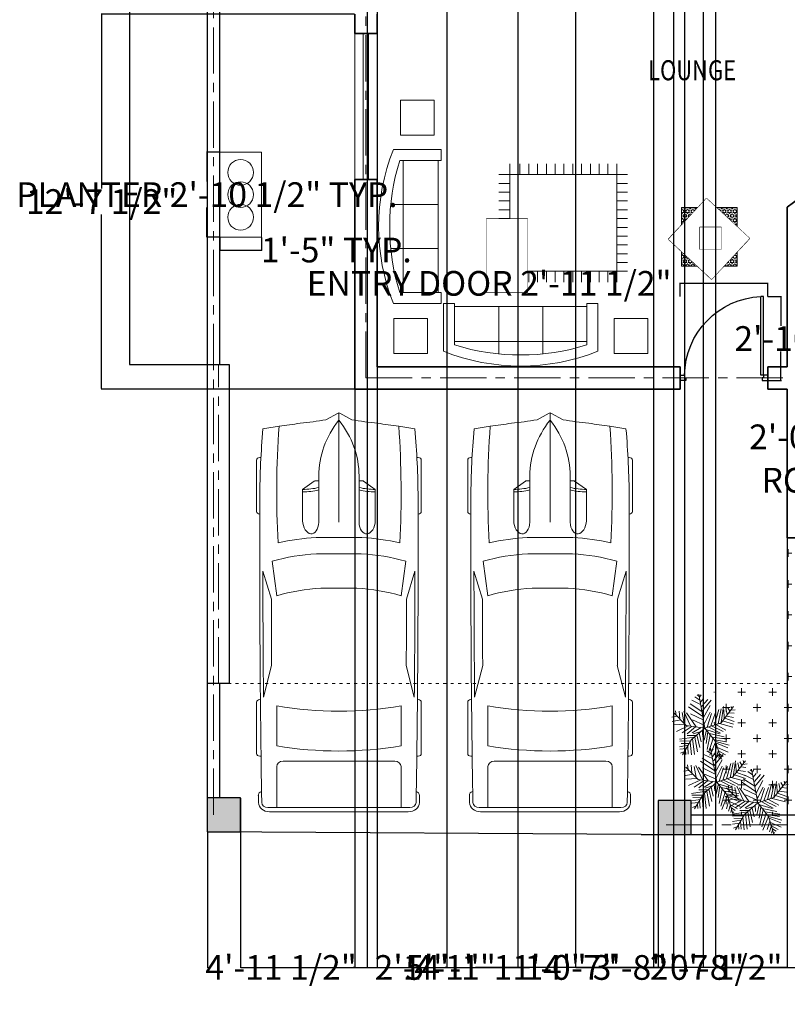
# Model space of a CAD drawing. Units: inches. Extents: x 541 to 1172, y -20 to 887.
# Tile 1 of 8: x 541 to 851, y -20 to 378. Entities that reach past the tile are written whole.
import ezdxf

# ---------------------------------------------------------------- set-up
doc = ezdxf.new("R2010")
doc.units = ezdxf.units.IN
doc.header["$MEASUREMENT"] = 0
doc.set_wipeout_variables(frame=1)
doc.linetypes.add('ACAD_ISO03W100', pattern=[30, 12, -18])
doc.linetypes.add('CENTER', pattern=[50.8, 31.75, -6.35, 6.35, -6.35])
doc.layers.get('0').update_dxf_attribs({"color": 70})
for name, color, linetype, lineweight in [('A-ANNO-DIMS', 2, 'Continuous', 18), ('A-AREA-IDEN', 7, 'Continuous', 20), ('A-DOOR', 4, 'Continuous', 25), ('A-FURN', 30, 'Continuous', 18), ('A-ROOF-OVHD', 8, 'ACAD_ISO03W100', 18), ('A-WALL-CNTR', 1, 'CENTER', 13), ('C-PKNG-VEHI', 8, 'Continuous', 18), ('C-PROP', 7, 'Continuous', 25), ('L-PLNT', 70, 'Continuous', 18), ('L-PLNT-PATT', 70, 'Continuous', 13), ('L-SITE-PATT', 252, 'Continuous', 13), ('L-SITE-WALL', 7, 'Continuous', 30), ('WALL', 7, 'Continuous', 35), ('WINDOW', 2, 'Continuous', 18)]:
    doc.layers.add(name, color=color, linetype=linetype, lineweight=lineweight)
doc.styles.get("Standard").update_dxf_attribs({"font": 'arial.ttf'})
doc.styles.add('YQ_DIM', font='SUPEROS.SHX', dxfattribs={"width": 0.8, "bigfont": 'HZDX.SHX'})
doc.dimstyles.get("Standard").update_dxf_attribs({"dimtxt": 10, "dimasz": 0.18, "dimexe": 0.18, "dimexo": 0.0625, "dimgap": 0.09, "dimtad": 0, "dimtih": 1, "dimtoh": 1, "dimdec": 1, "dimzin": 0, "dimdsep": 46, "dimlunit": 4, "dimtxsty": 'Standard', "dimcen": 0.09, "dimadec": 0, "dimazin": 0, "dimtfac": 1, "dimtdec": 1, "dimtofl": 0, "dimtmove": 0, "dimatfit": 3, "dimfxl": 1, "dimtolj": 1, "dimtzin": 0, "dimarcsym": 0})

# ---------------------------------------------------------------- blocks, each defined once
blk = doc.blocks.new('*D3')
at = {"layer": 'A-ANNO-DIMS', "color": 0, "lineweight": -2, "transparency": 16777216}
for p, q in [((616.57, 829.68), (585.07, 829.68)), ((585.25, 829.5), (585.25, 539.38)), ((585.25, 238.86), (585.25, 528.98)), ((621.57, 238.68), (585.07, 238.68))]:
    blk.add_line(p, q, dxfattribs=at)
for points in [[(585.22, 829.5), (585.28, 829.5), (585.25, 829.68)], [(585.22, 238.86), (585.28, 238.86), (585.25, 238.68)]]:
    blk.add_solid(points, dxfattribs=at)
at = {"layer": 'Defpoints', "color": 0, "lineweight": -2, "transparency": 16777216}
for p in [(616.64, 829.68), (585.25, 238.68), (621.64, 238.68)]:
    blk.add_point(p, dxfattribs=at)
at = {"layer": 'A-ANNO-DIMS', "color": 0, "transparency": 16777216, "insert": (585.25, 534.18), "char_height": 10, "attachment_point": 5}
blk.add_mtext('\\A1;49\'-3"', dxfattribs=at)
blk = doc.blocks.new('*U5')
for p, q in [((21.1, 37.41), (21.1, 36.83)), ((46.55, 38.89), (22.35, 38.89)), ((47.8, 37.39), (47.8, 37.41)), ((135.45, 37.07), (135.45, 37.41)), ((136.7, 38.89), (160.9, 38.89)), ((162.15, 37.41), (162.15, 36.77)), ((87.99, 31.87), (74.76, 35.92)), ((134.31, 35.6), (119.29, 31.78)), ((186.47, -33.5), (186.47, 33.5)), ((188.4, -32.76), (188.4, 32.76)), ((70.03, 31.54), (86.41, 29.35)), ((138.42, 29.35), (157.25, 29.35)), ((186.47, 29.35), (167.01, 29.35)), ((164.52, 26.39), (164.52, -26.39)), ((32.27, 11.63), (36.13, 17.17)), ((36.13, 17.17), (50.94, 17.17)), ((29.77, 9.51), (51.68, 9.51)), ((32.12, 9.51), (32.12, 11.15)), ((58.92, -10.77), (58.92, 10.77)), ((66.55, -10.53), (66.55, 10.53)), ((186.47, -10.53), (186.47, 10.53)), ((3.27, 6.13), (0.1, 0.41)), ((82.74, 8.5), (82.74, -8.5)), ((0, 0), (51.68, 0)), ((0.1, -0.41), (3.27, -6.13)), ((29.77, -9.51), (51.68, -9.51)), ((32.12, -9.51), (32.12, -11.15)), ((32.27, -11.63), (36.13, -17.17)), ((36.13, -17.17), (50.94, -17.17)), ((86.41, -29.35), (70.03, -31.54)), ((87.99, -31.87), (74.76, -35.92)), ((134.31, -35.6), (119.29, -31.78)), ((157.25, -29.35), (138.42, -29.35)), ((167.01, -29.35), (186.47, -29.35)), ((21.1, -37.41), (21.1, -36.83)), ((135.45, -37.07), (135.45, -37.41)), ((162.15, -37.41), (162.15, -36.77)), ((46.55, -38.89), (22.35, -38.89)), ((47.8, -37.39), (47.8, -37.41)), ((136.7, -38.89), (160.9, -38.89))]:
    blk.add_line(p, q)
for centre, major_axis, ratio, start_param, end_param in [((41.19, -490.86), (0, 528.23), 0.842304, 0.00281, 0.075598), ((22.35, 37.41), (0, -1.48), 0.842304, 3.141593, 4.712389), ((64.48, -10555.62), (0, 10593.03), 0.842304, -0.013397, 0.002797), ((46.55, 37.41), (0, 1.48), 0.842304, -1.570796, 0), ((136.7, 37.41), (0, -1.48), 0.842304, 3.141593, 4.712389), ((160.9, 37.41), (0, 1.48), 0.842304, -1.570796, 0), ((180.63, 35.84), (0, 2.22), 0.842304, -0.013017, 1.249894), ((64.48, -10556.36), (0, 10595.31), 0.842304, -0.013397, -0.013017), ((183.98, 32.76), (0, -5.25), 0.842304, 1.570796, 3.128196), ((266.03, -27.52), (0, 313.31), 0.842304, 1.367076, 1.39176), ((64.48, -10555.62), (0, -10591.55), 0.842304, 3.133765, 3.140441), ((183.98, 33.5), (0, -2.96), 0.842304, 1.570796, 3.128196), ((259.18, -27.52), (0, -305.3), 0.842304, 4.528606, 4.561838), ((37.47, -593.96), (0, -623.33), 0.842304, 3.096046, 3.200911), ((134.4, 5.39), (0, -89.78), 0.842304, 4.449482, 4.652344), ((135.29, 5.39), (0, 81.77), 0.842304, 1.245306, 1.50788), ((149.6, 2.8), (0, -79.58), 0.842304, 4.372215, 4.640744), ((95.79, -3666.35), (0, -3698.24), 0.842304, 3.134049, 3.144098), ((17.08, 0), (0, 147.02), 0.842304, 4.511394, 4.913384), ((35.91, 0), (0, 147.02), 0.842304, 4.511394, 4.913384), ((167.01, 26.39), (0, 2.96), 0.842304, 0, 1.570796), ((-204.49, 52.4), (0, -250.96), 0.842304, 1.385369, 1.434372), ((13.04, 17.01), (0, 27.42), 0.842304, 4.435146, 4.718221), ((14.2, 17.01), (0, 27.42), 0.842304, 4.435146, 4.718221), ((50.79, 13.34), (6.34, -0.36), 0.603834, -1.395552, 1.581315), ((29.77, -46.66), (0, 56.17), 0.842304, 0, 0.590319), ((32.75, 11.15), (0, 0.74), 0.842304, 0.879714, 1.570796), ((0.62, 0), (0, -0.74), 0.842304, 4.131459, 5.293319), ((29.77, 46.66), (0, 56.17), 0.842304, 2.551274, 3.141593), ((-204.49, -52.4), (0, 250.96), 0.842304, -1.434372, -1.385369), ((149.6, -2.8), (0, -79.58), 0.842304, -1.499151, -1.230623), ((32.75, -11.15), (0, -0.74), 0.842304, 4.712389, 5.403472), ((13.04, -17.01), (0, -27.42), 0.842304, 1.564964, 1.848039), ((14.2, -17.01), (0, -27.42), 0.842304, 1.564964, 1.848039), ((134.4, -5.39), (0, -89.78), 0.842304, -1.510751, -1.307889), ((135.29, -5.39), (0, -81.77), 0.842304, -1.50788, -1.245306), ((259.18, 27.52), (0, 305.3), 0.842304, 1.721348, 1.754579), ((167.01, -26.39), (0, -2.96), 0.842304, 4.712389, 6.283185), ((266.03, 27.52), (0, 313.31), 0.842304, 1.749832, 1.774517), ((37.47, 593.96), (0, -623.33), 0.842304, -0.059319, 0.045547), ((95.79, 3666.35), (0, -3698.24), 0.842304, -0.002505, 0.007544), ((41.19, 490.86), (0, -528.23), 0.842304, -0.075598, -0.00281), ((64.48, 10555.62), (0, 10593.03), 0.842304, 3.138796, 3.15499), ((64.48, 10555.62), (0, -10591.55), 0.842304, 0.001152, 0.007828), ((180.63, -35.84), (0, -2.22), 0.842304, -1.249894, 0.013017), ((183.98, -33.5), (0, 2.96), 0.842304, 3.15499, 4.712389), ((183.98, -32.76), (0, -5.25), 0.842304, 0.013397, 1.570796), ((22.35, -37.41), (0, 1.48), 0.842304, 1.570796, 3.141593), ((46.55, -37.41), (0, -1.48), 0.842304, 0, 1.570796), ((136.7, -37.41), (0, -1.48), 0.842304, -1.570796, 0), ((160.9, -37.41), (0, 1.48), 0.842304, 3.141593, 4.712389), ((64.48, 10556.36), (0, 10595.31), 0.842304, 3.15461, 3.15499)]:
    blk.add_ellipse(centre, major_axis=major_axis, ratio=ratio, start_param=start_param, end_param=end_param)
at = {"extrusion": (0, 0, -1)}
blk.add_ellipse((50.79, -13.34), major_axis=(6.34, 0.36), ratio=0.603834, start_param=-1.395552, end_param=1.581315, dxfattribs=at)
blk = doc.blocks.new('*U7')
for p, q in [((-8.737, 47.138), (-17.069, 52.711)), ((-10.186, 53.64), (-13.084, 55.962)), ((0, 0), (-10.5, 57)), ((-9.099, 51.782), (-6.563, 55.962)), ((-3.665, 19.273), (-27.574, 35.527)), ((-5.114, 28.097), (-24.676, 40.636)), ((-7.288, 39.707), (-21.778, 46.673)), ((-7.65, 43.423), (-2.578, 49.46)), ((-5.839, 35.992), (4.667, 48.067)), ((-5.114, 27.632), (10.463, 46.673)), ((-2.941, 16.486), (8.652, 37.85)), ((27, 9), (48, 36)), ((27.127, 9.056), (31.112, 35.992)), ((38.719, 34.134), (41.979, 28.561)), ((44.153, 36.456), (45.239, 32.741)), ((-47.498, 19.737), (-55.83, 18.344)), ((-31.5, 4.5), (-52.5, 25.5)), ((-48.585, 21.131), (-49.309, 29.026)), ((-43.513, 28.561), (-42.427, 15.558)), ((-38.442, 26.239), (-34.819, 7.663)), ((-35.544, 28.097), (-24.314, 3.947)), ((-14.533, 2.09), (-30.834, 25.31)), ((-24.314, 23.917), (-2.941, 13.7)), ((-1.129, 6.734), (9.014, 26.704)), ((3.942, 1.625), (11.187, 24.381)), ((10.101, 3.483), (17.708, 26.239)), ((16.259, 5.805), (23.142, 31.348)), ((22.055, 7.198), (27.489, 32.277)), ((31.836, 30.883), (32.561, 16.486)), ((35.096, 32.741), (37.27, 22.524)), ((36.183, 19.737), (48.137, 17.88)), ((40.53, 25.775), (48.862, 24.846)), ((43.791, 29.954), (51.036, 30.883)), ((-40.615, 13.7), (-55.105, 10.913)), ((-33.37, 6.269), (-52.207, 5.34)), ((-28.299, 3.483), (-47.86, -5.805)), ((-21.416, 3.018), (-38.079, -8.128)), ((0, 0), (-31.5, 4.5)), ((-15.982, 2.09), (-30.11, -9.521)), ((0, 0), (-22.5, -19.5)), ((-6.563, 1.161), (-21.416, -8.128)), ((-20.691, 13.7), (-1.129, 4.876)), ((0, 0), (27, 9)), ((0, 0), (18, -22.5)), ((6.478, 1.625), (26.04, -8.592)), ((11.187, 3.483), (30.749, -5.805)), ((18.07, 5.805), (35.096, -3.483)), ((24.229, 7.663), (46.688, 1.625)), ((29.662, 12.307), (48.137, 6.269)), ((33.285, 16.486), (48.862, 10.913)), ((-17.431, -15.094), (-42.789, -18.809)), ((-15.257, -12.772), (-30.11, -12.772)), ((-6.563, -5.805), (-19.967, -9.985)), ((-17.069, -15.094), (-12.721, -40.172)), ((-13.446, -11.378), (-8.737, -32.741)), ((-9.461, -8.592), (-6.201, -23.453)), ((-4.752, -3.483), (-3.665, -14.629)), ((2.493, -3.019), (-1.491, -20.202)), ((1.769, -2.555), (24.229, -9.521)), ((5.029, -6.27), (2.131, -25.775)), ((9.014, -11.378), (3.58, -35.992)), ((7.565, -9.056), (32.198, -14.629)), ((12.274, -15.094), (36.907, -18.809)), ((-28.299, -29.026), (-42.789, -31.348)), ((-24.314, -21.596), (-42.427, -22.06)), ((-26.849, -26.24), (-40.253, -25.775)), ((-22.5, -19.5), (-37.5, -45)), ((-29.023, -30.884), (-27.936, -43.887)), ((-25.038, -23.918), (-22.865, -45.281)), ((-20.691, -18.345), (-17.793, -44.352)), ((14.085, -16.951), (6.478, -40.172)), ((18.07, -22.524), (8.289, -45.745)), ((20.244, -30.419), (15.897, -44.816)), ((16.259, -19.738), (36.183, -22.989)), ((18, -22.5), (27, -52.5)), ((18.433, -22.524), (40.53, -29.026)), ((19.157, -25.311), (38.719, -33.206)), ((21.331, -32.741), (39.081, -40.636)), ((-30.834, -34.135), (-42.427, -35.528)), ((-34.457, -39.708), (-40.978, -42.494)), ((-32.646, -36.921), (-31.921, -44.352)), ((22.78, -37.85), (19.519, -48.532)), ((22.78, -38.314), (34.372, -44.816)), ((24.591, -45.745), (23.142, -50.854)), ((24.591, -43.423), (30.749, -47.603)), ((26.764, -49.925), (28.213, -50.854))]:
    blk.add_line(p, q)
blk = doc.blocks.new('Sofa - Roundback 7 ft.')
for p, q in [((-12.00002, -32.4421), (-12.00003, -6.5971)), ((11.99997, -32.4421), (11.99998, -6.5971)), ((-36.000027, -34), (-36.000027, -11.4696)), ((-35.999844, -13.3819), (35.9998, -13.3819)), ((35.99998, -34), (35.99998, -11.4696)), ((-36.000027, -32.4421), (35.99998, -32.4421))]:
    blk.add_line(p, q)
for points in [[(-36.000027, -34), (-42.000027, -34), (-42.000027, -8)], [(41.99998, -8), (41.99998, -34), (35.99998, -34)]]:
    blk.add_lwpolyline(points)
for centre, radius, start, end in [((0, -114.25), 114.25, 68.43141, 111.5686), ((-0.00001, -127.1968), 121.1968, 72.72033, 107.2797)]:
    blk.add_arc(centre, radius, start, end)
blk = doc.blocks.new('DR_D01')
at = {"lineweight": -2}
for p, q in [((-0.45, 0.93), (-0.42, 0.93)), ((-0.45, 0.03), (-0.45, 0.93)), ((-0.42, 0.03), (-0.42, 0.93)), ((-0.5, 0.03), (-0.42, 0.03)), ((-0.5, 0.03), (-0.5, -0.03)), ((-0.45, 0.03), (-0.45, 0)), ((-0.45, 0), (-0.435, 0)), ((-0.435, 0), (-0.435, -0.03)), ((0.435, 0), (0.435, -0.03)), ((0.45, 0), (0.435, 0)), ((0.45, 0.03), (0.45, 0)), ((0.5, 0.03), (0.45, 0.03)), ((0.5, -0.03), (0.5, 0.03)), ((-0.435, -0.03), (-0.5, -0.03)), ((0.435, -0.03), (0.5, -0.03))]:
    blk.add_line(p, q, dxfattribs=at)
blk.add_arc((-0.46, 0.021), 0.91, 0.5915, 87.4664, dxfattribs=at)
blk = doc.blocks.new('WD_WIN4')
at = {"lineweight": -2}
for p, q in [((-0.5, 0.5), (0.5, 0.5)), ((-0.5, 0.12), (0.5, 0.12)), ((-0.5, -0.12), (0.5, -0.12)), ((-0.5, -0.5), (0.5, -0.5))]:
    blk.add_line(p, q, dxfattribs=at)
blk = doc.blocks.new('PLANTER-THREE-ROUND')
blk.add_lwpolyline([(34.49, 16.89), (0, 16.89), (0, 0), (34.49, 0)], close=True)
for centre in [(8.25, 8.45), (17.25, 8.45), (26.39, 8.45)]:
    blk.add_circle(centre, 5.21)
blk = doc.blocks.new('RUG-FRINGED-WITH-LOW-TABLE')
for p, q in [((4.37, 52.04), (4.37, 47.68)), ((7.93, 52.04), (7.93, 47.68)), ((11.48, 52.04), (11.48, 47.68)), ((15.04, 52.04), (15.04, 47.68)), ((18.6, 52.04), (18.6, 47.68)), ((22.16, 52.04), (22.16, 47.68)), ((25.72, 52.04), (25.72, 47.68)), ((29.27, 52.04), (29.27, 47.68)), ((32.83, 52.04), (32.83, 47.68)), ((36.39, 52.04), (36.39, 47.68)), ((39.95, 52.04), (39.95, 47.68)), ((43.51, 52.04), (43.51, 47.68)), ((47.65, 52.04), (47.65, 47.68)), ((4.37, 47.68), (0, 47.68)), ((4.37, 44.12), (0, 44.12)), ((47.65, 47.68), (52.02, 47.68)), ((47.65, 44.12), (52.02, 44.12)), ((4.37, 40.56), (0, 40.56)), ((47.65, 40.56), (52.02, 40.56)), ((4.37, 37), (0, 37)), ((47.65, 37), (52.02, 37)), ((4.37, 33.44), (0, 33.44)), ((47.65, 33.44), (52.02, 33.44)), ((4.37, 29.89), (0, 29.89)), ((47.65, 29.89), (52.02, 29.89)), ((4.37, 26.33), (0, 26.33)), ((47.65, 26.33), (52.02, 26.33)), ((4.37, 22.77), (0, 22.77)), ((47.65, 22.77), (52.02, 22.77)), ((4.37, 19.21), (0, 19.21)), ((47.65, 19.21), (52.02, 19.21)), ((4.37, 15.65), (0, 15.65)), ((4.37, 12.1), (0, 12.1)), ((47.65, 15.65), (52.02, 15.65)), ((47.65, 12.1), (52.02, 12.1)), ((4.37, 8.54), (0, 8.54)), ((4.37, 4.17), (4.37, 8.54)), ((7.93, 4.17), (7.93, 8.54)), ((11.48, 4.17), (11.48, 8.54)), ((15.04, 4.17), (15.04, 8.54)), ((18.6, 4.17), (18.6, 8.54)), ((22.16, 4.17), (22.16, 8.54)), ((25.72, 4.17), (25.72, 8.54)), ((29.27, 4.17), (29.27, 8.54)), ((32.83, 4.17), (32.83, 8.54)), ((36.39, 4.17), (36.39, 8.54)), ((39.95, 4.17), (39.95, 8.54)), ((43.51, 4.17), (43.51, 8.54)), ((47.65, 8.54), (52.02, 8.54)), ((47.65, 4.17), (47.65, 8.54))]:
    blk.add_line(p, q)
for points in [[(4.37, 47.68), (47.65, 47.68), (47.65, 8.54), (4.37, 8.54)], [(40.42, 29.74), (57.09, 29.74), (57.09, 0), (40.42, 0)]]:
    blk.add_lwpolyline(points, close=True)
blk.add_wipeout([(57.09, 0), (40.42, 0), (40.42, 29.74), (57.09, 29.74), (57.09, 29.74)])
blk = doc.blocks.new('FURN-ACCENT-SQUARE')
h = blk.add_hatch()
h.set_pattern_fill('STARS', color=256, scale=4.255607)
h.set_pattern_definition([(0, (-199.5324, -51.5532), (0, 0.921366), [0.531951, -0.531951]), (60, (-199.5324, -51.5532), (-0.7979263, 0.460683), [0.531951, -0.531951]), (120, (-199.2664, -51.0925), (-0.7979263, -0.460683), [0.531951, -0.531951])])
h.paths.add_polyline_path([(27.75, 29.01), (5.18, 29.01), (5.18, 5.24), (27.75, 5.24)])
for points in [[(0, 16.17), (15.35, 32.72), (32.78, 16.55), (17.43, 0)], [(5.18, 29.01), (27.75, 29.01), (27.75, 5.24), (5.18, 5.24)]]:
    blk.add_lwpolyline(points, close=True)
blk.add_wipeout([(32.78, 16.55), (17.43, 0), (0, 16.17), (15.35, 32.72)])
blk.add_lwpolyline([(12.67, 21.04), (21.3, 21.04), (21.3, 12.15), (12.67, 12.15)], close=True)
blk.add_wipeout([(21.3, 12.15), (12.67, 12.15), (12.67, 21.04), (21.3, 21.04), (21.3, 21.04)])
blk = doc.blocks.new('FURN-END-TABLE')
blk.add_lwpolyline([(0, 14.11), (13.62, 14.11), (13.62, 0), (0, 0)], close=True)
blk = doc.blocks.new('*D43')
at = {"layer": 'A-ANNO-DIMS', "color": 0, "lineweight": -2, "transparency": 16777216}
for p, q in [((621.57, 324.84), (616.28, 324.84)), ((616.46, 324.66), (616.46, 312.86)), ((616.46, 290.53), (616.46, 302.34)), ((621.57, 290.35), (616.28, 290.35))]:
    blk.add_line(p, q, dxfattribs=at)
for points in [[(616.43, 324.66), (616.49, 324.66), (616.46, 324.84)], [(616.43, 290.53), (616.49, 290.53), (616.46, 290.35)]]:
    blk.add_solid(points, dxfattribs=at)
at = {"layer": 'Defpoints', "color": 0, "lineweight": -2, "transparency": 16777216}
for p in [(621.64, 324.84), (616.46, 290.35), (621.64, 290.35)]:
    blk.add_point(p, dxfattribs=at)
at = {"layer": 'A-ANNO-DIMS', "color": 0, "transparency": 16777216, "insert": (616.46, 307.6), "char_height": 10, "attachment_point": 5}
blk.add_mtext('\\A1;PLANTER 2\'-10 1/2" TYP.', dxfattribs=at)
blk = doc.blocks.new('*D44')
at = {"layer": 'A-ANNO-DIMS', "color": 0, "lineweight": -2, "transparency": 16777216}
for p, q in [((621.64, 290.29), (621.64, 285)), ((638.53, 290.29), (638.53, 285)), ((621.82, 285.18), (638.35, 285.18)), ((638.53, 285.18), (638.71, 285.18))]:
    blk.add_line(p, q, dxfattribs=at)
for points in [[(621.82, 285.21), (621.82, 285.15), (621.64, 285.18)], [(638.35, 285.21), (638.35, 285.15), (638.53, 285.18)]]:
    blk.add_solid(points, dxfattribs=at)
at = {"layer": 'Defpoints', "color": 0, "lineweight": -2, "transparency": 16777216}
for p in [(621.64, 290.35), (638.53, 290.35), (638.53, 285.18)]:
    blk.add_point(p, dxfattribs=at)
at = {"layer": 'A-ANNO-DIMS', "color": 0, "transparency": 16777216, "insert": (668.8, 285.18), "char_height": 10, "attachment_point": 5}
blk.add_mtext('\\A1;1\'-5" TYP.', dxfattribs=at)
blk = doc.blocks.new('*D63')
at = {"layer": 'A-ANNO-DIMS', "color": 0, "lineweight": -2, "transparency": 16777216}
for p, q in [((887.91, 205.52), (883.75, 205.52)), ((883.93, 205.34), (883.93, 197.29)), ((883.93, 178.7), (883.93, 186.75)), ((887.91, 178.52), (883.75, 178.52))]:
    blk.add_line(p, q, dxfattribs=at)
for points in [[(883.9, 205.34), (883.96, 205.34), (883.93, 205.52)], [(883.9, 178.7), (883.96, 178.7), (883.93, 178.52)]]:
    blk.add_solid(points, dxfattribs=at)
at = {"layer": 'Defpoints', "color": 0, "lineweight": -2, "transparency": 16777216}
for p in [(887.98, 205.52), (883.93, 178.52), (887.98, 178.52)]:
    blk.add_point(p, dxfattribs=at)
at = {"layer": 'A-ANNO-DIMS', "color": 0, "transparency": 16777216, "insert": (883.93, 192.02), "char_height": 10, "attachment_point": 5}
blk.add_mtext('\\A1;ROCKER 2\'-3"', dxfattribs=at)
blk = doc.blocks.new('*D64')
at = {"layer": 'A-ANNO-DIMS', "color": 0, "lineweight": -2, "transparency": 16777216}
for p, q in [((887.98, 209.57), (887.8, 209.57)), ((887.98, 205.58), (887.98, 209.75)), ((912.23, 209.57), (888.16, 209.57)), ((912.41, 205.58), (912.41, 209.75))]:
    blk.add_line(p, q, dxfattribs=at)
for points in [[(888.16, 209.6), (888.16, 209.54), (887.98, 209.57)], [(912.23, 209.6), (912.23, 209.54), (912.41, 209.57)]]:
    blk.add_solid(points, dxfattribs=at)
at = {"layer": 'Defpoints', "color": 0, "lineweight": -2, "transparency": 16777216}
for p in [(887.98, 209.57), (887.98, 205.52), (912.41, 205.52)]:
    blk.add_point(p, dxfattribs=at)
at = {"layer": 'A-ANNO-DIMS', "color": 0, "transparency": 16777216, "insert": (862.68, 209.57), "char_height": 10, "attachment_point": 5}
blk.add_mtext('\\A1;2\'-0 1/2"', dxfattribs=at)
blk = doc.blocks.new('*D67')
at = {"layer": 'A-ANNO-DIMS', "color": 0, "lineweight": -2, "transparency": 16777216}
for p, q in [((807.98, 271.69), (807.8, 271.69)), ((807.98, 266.43), (807.98, 271.87)), ((843.23, 271.69), (808.16, 271.69)), ((843.41, 266.43), (843.41, 271.87))]:
    blk.add_line(p, q, dxfattribs=at)
for points in [[(808.16, 271.72), (808.16, 271.66), (807.98, 271.69)], [(843.23, 271.72), (843.23, 271.66), (843.41, 271.69)]]:
    blk.add_solid(points, dxfattribs=at)
at = {"layer": 'Defpoints', "color": 0, "lineweight": -2, "transparency": 16777216}
for p in [(807.98, 271.69), (807.98, 266.37), (843.41, 266.37)]:
    blk.add_point(p, dxfattribs=at)
at = {"layer": 'A-ANNO-DIMS', "color": 0, "transparency": 16777216, "insert": (730.63, 271.69), "char_height": 10, "attachment_point": 5}
blk.add_mtext('\\A1;ENTRY DOOR 2\'-11 1/2"', dxfattribs=at)
blk = doc.blocks.new('*D68')
at = {"layer": 'A-ANNO-DIMS', "color": 0, "lineweight": -2, "transparency": 16777216}
for p, q in [((843.47, 266.37), (848.9, 266.37)), ((848.72, 266.19), (848.72, 254.56)), ((848.72, 232.53), (848.72, 244.17)), ((843.47, 232.35), (848.9, 232.35))]:
    blk.add_line(p, q, dxfattribs=at)
for points in [[(848.69, 266.19), (848.75, 266.19), (848.72, 266.37)], [(848.69, 232.53), (848.75, 232.53), (848.72, 232.35)]]:
    blk.add_solid(points, dxfattribs=at)
at = {"layer": 'Defpoints', "color": 0, "lineweight": -2, "transparency": 16777216}
for p in [(843.41, 266.37), (848.72, 266.37), (843.41, 232.35)]:
    blk.add_point(p, dxfattribs=at)
at = {"layer": 'A-ANNO-DIMS', "color": 0, "transparency": 16777216, "insert": (848.72, 249.36), "char_height": 10, "attachment_point": 5}
blk.add_mtext('\\A1;2\'-10"', dxfattribs=at)
blk = doc.blocks.new('*D71')
at = {"layer": 'A-ANNO-DIMS', "color": 0, "lineweight": -2, "transparency": 16777216}
for p, q in [((676.28, 228.86), (676.28, -5.37)), ((616.64, 49.62), (616.64, -5.37)), ((616.82, -5.19), (617.34, -5.19)), ((676.1, -5.19), (675.58, -5.19))]:
    blk.add_line(p, q, dxfattribs=at)
for points in [[(616.82, -5.16), (616.82, -5.22), (616.64, -5.19)], [(676.1, -5.16), (676.1, -5.22), (676.28, -5.19)]]:
    blk.add_solid(points, dxfattribs=at)
at = {"layer": 'Defpoints', "color": 0, "lineweight": -2, "transparency": 16777216}
for p in [(676.28, 228.92), (616.64, 49.68), (676.28, -5.19)]:
    blk.add_point(p, dxfattribs=at)
at = {"layer": 'A-ANNO-DIMS', "color": 0, "transparency": 16777216, "insert": (646.46, -5.19), "char_height": 10, "attachment_point": 5}
blk.add_mtext('\\A1;4\'-11 1/2"', dxfattribs=at)
blk = doc.blocks.new('*D72')
at = {"layer": 'A-ANNO-DIMS', "color": 0, "lineweight": -2, "transparency": 16777216}
for p, q in [((676.28, 228.86), (676.28, -5.37)), ((851.28, 228.86), (851.28, -5.37)), ((676.46, -5.19), (746.99, -5.19)), ((851.1, -5.19), (780.58, -5.19))]:
    blk.add_line(p, q, dxfattribs=at)
for points in [[(676.46, -5.16), (676.46, -5.22), (676.28, -5.19)], [(851.1, -5.16), (851.1, -5.22), (851.28, -5.19)]]:
    blk.add_solid(points, dxfattribs=at)
at = {"layer": 'Defpoints', "color": 0, "lineweight": -2, "transparency": 16777216}
for p in [(676.28, 228.92), (851.28, 228.92), (851.28, -5.19)]:
    blk.add_point(p, dxfattribs=at)
at = {"layer": 'A-ANNO-DIMS', "color": 0, "transparency": 16777216, "insert": (763.78, -5.19), "char_height": 10, "attachment_point": 5}
blk.add_mtext('\\A1;14\'-7"', dxfattribs=at)
blk = doc.blocks.new('*D74')
at = {"layer": 'A-ANNO-DIMS', "color": 0, "lineweight": -2, "transparency": 16777216}
for p, q in [((629.99, 63.37), (629.99, -5.37)), ((799.03, 62.34), (799.03, -5.37)), ((630.17, -5.19), (697.71, -5.19)), ((798.85, -5.19), (731.3, -5.19))]:
    blk.add_line(p, q, dxfattribs=at)
for points in [[(630.17, -5.16), (630.17, -5.22), (629.99, -5.19)], [(798.85, -5.16), (798.85, -5.22), (799.03, -5.19)]]:
    blk.add_solid(points, dxfattribs=at)
at = {"layer": 'Defpoints', "color": 0, "lineweight": -2, "transparency": 16777216}
for p in [(629.99, 63.43), (799.03, 62.4), (799.03, -5.19)]:
    blk.add_point(p, dxfattribs=at)
at = {"layer": 'A-ANNO-DIMS', "color": 0, "transparency": 16777216, "insert": (714.51, -5.19), "char_height": 10, "attachment_point": 5}
blk.add_mtext('\\A1;14\'-1"', dxfattribs=at)
blk = doc.blocks.new('*D82')
at = {"layer": 'A-ANNO-DIMS', "color": 0, "lineweight": -2, "transparency": 16777216}
for p, q in [((681.28, 586.59), (681.28, -5.37)), ((742.28, 526.59), (742.28, -5.37)), ((681.46, -5.19), (698.4, -5.19)), ((742.1, -5.19), (725.16, -5.19))]:
    blk.add_line(p, q, dxfattribs=at)
for points in [[(681.46, -5.16), (681.46, -5.22), (681.28, -5.19)], [(742.1, -5.16), (742.1, -5.22), (742.28, -5.19)]]:
    blk.add_solid(points, dxfattribs=at)
at = {"layer": 'Defpoints', "color": 0, "lineweight": -2, "transparency": 16777216}
for p in [(681.28, 586.65), (742.28, 526.65), (742.28, -5.19)]:
    blk.add_point(p, dxfattribs=at)
at = {"layer": 'A-ANNO-DIMS', "color": 0, "transparency": 16777216, "insert": (711.78, -5.19), "char_height": 10, "attachment_point": 5}
blk.add_mtext('\\A1;5\'-1"', dxfattribs=at)
blk = doc.blocks.new('*D84')
at = {"layer": 'A-ANNO-DIMS', "color": 0, "lineweight": -2, "transparency": 16777216}
for p, q in [((685.28, 389.59), (685.28, -5.37)), ((817.28, 389.59), (817.28, -5.37)), ((685.46, -5.19), (734.49, -5.19)), ((817.1, -5.19), (768.08, -5.19))]:
    blk.add_line(p, q, dxfattribs=at)
for points in [[(685.46, -5.16), (685.46, -5.22), (685.28, -5.19)], [(817.1, -5.16), (817.1, -5.22), (817.28, -5.19)]]:
    blk.add_solid(points, dxfattribs=at)
at = {"layer": 'Defpoints', "color": 0, "lineweight": -2, "transparency": 16777216}
for p in [(685.28, 389.65), (817.28, 389.65), (817.28, -5.19)]:
    blk.add_point(p, dxfattribs=at)
at = {"layer": 'A-ANNO-DIMS', "color": 0, "transparency": 16777216, "insert": (751.28, -5.19), "char_height": 10, "attachment_point": 5}
blk.add_mtext('\\A1;11\'-0"', dxfattribs=at)
blk = doc.blocks.new('*D92')
at = {"layer": 'A-ANNO-DIMS', "color": 0, "lineweight": -2, "transparency": 16777216}
for p, q in [((676.22, 380.65), (573.66, 380.65)), ((573.84, 380.47), (573.84, 310.05)), ((573.84, 229.1), (573.84, 299.53)), ((676.22, 228.92), (573.66, 228.92))]:
    blk.add_line(p, q, dxfattribs=at)
for points in [[(573.81, 380.47), (573.87, 380.47), (573.84, 380.65)], [(573.81, 229.1), (573.87, 229.1), (573.84, 228.92)]]:
    blk.add_solid(points, dxfattribs=at)
at = {"layer": 'Defpoints', "color": 0, "lineweight": -2, "transparency": 16777216}
for p in [(573.84, 380.65), (676.28, 380.65), (676.28, 228.92)]:
    blk.add_point(p, dxfattribs=at)
at = {"layer": 'A-ANNO-DIMS', "color": 0, "transparency": 16777216, "insert": (573.84, 304.79), "char_height": 10, "attachment_point": 5}
blk.add_mtext('\\A1;12\'-7 1/2"', dxfattribs=at)
blk = doc.blocks.new('*D99')
at = {"layer": 'A-ANNO-DIMS', "color": 0, "lineweight": -2, "transparency": 16777216}
for p, q in [((765.53, 591.59), (765.53, -5.37)), ((797.19, 591.59), (797.19, -5.37)), ((765.71, -5.19), (797.01, -5.19)), ((797.19, -5.19), (797.37, -5.19))]:
    blk.add_line(p, q, dxfattribs=at)
for points in [[(765.71, -5.16), (765.71, -5.22), (765.53, -5.19)], [(797.01, -5.16), (797.01, -5.22), (797.19, -5.19)]]:
    blk.add_solid(points, dxfattribs=at)
at = {"layer": 'Defpoints', "color": 0, "lineweight": -2, "transparency": 16777216}
for p in [(765.53, 591.65), (797.19, 591.65), (797.19, -5.19)]:
    blk.add_point(p, dxfattribs=at)
at = {"layer": 'A-ANNO-DIMS', "color": 0, "transparency": 16777216, "insert": (822.49, -5.19), "char_height": 10, "attachment_point": 5}
blk.add_mtext('\\A1;2\'-7 1/2"', dxfattribs=at)
blk = doc.blocks.new('*D102')
at = {"layer": 'A-ANNO-DIMS', "color": 0, "lineweight": -2, "transparency": 16777216}
for p, q in [((822.26, 582.59), (822.26, -5.37)), ((866.83, 582.59), (866.83, -5.37)), ((822.44, -5.19), (866.65, -5.19)), ((866.83, -5.19), (867.01, -5.19))]:
    blk.add_line(p, q, dxfattribs=at)
for points in [[(822.44, -5.16), (822.44, -5.22), (822.26, -5.19)], [(866.65, -5.16), (866.65, -5.22), (866.83, -5.19)]]:
    blk.add_solid(points, dxfattribs=at)
at = {"layer": 'Defpoints', "color": 0, "lineweight": -2, "transparency": 16777216}
for p in [(822.26, 582.65), (866.83, 582.65), (866.83, -5.19)]:
    blk.add_point(p, dxfattribs=at)
at = {"layer": 'A-ANNO-DIMS', "color": 0, "transparency": 16777216, "insert": (892.04, -5.19), "char_height": 10, "attachment_point": 5}
blk.add_mtext('\\A1;3\'-8 1/2"', dxfattribs=at)
blk = doc.blocks.new('*D105')
at = {"layer": 'A-ANNO-DIMS', "color": 0, "lineweight": -2, "transparency": 16777216}
for p, q in [((797.19, 591.59), (797.19, -5.37)), ((805.28, 591.59), (805.28, -5.37)), ((797.37, -5.19), (805.1, -5.19)), ((805.28, -5.19), (805.46, -5.19))]:
    blk.add_line(p, q, dxfattribs=at)
for points in [[(797.37, -5.16), (797.37, -5.22), (797.19, -5.19)], [(805.1, -5.16), (805.1, -5.22), (805.28, -5.19)]]:
    blk.add_solid(points, dxfattribs=at)
at = {"layer": 'Defpoints', "color": 0, "lineweight": -2, "transparency": 16777216}
for p in [(797.19, 591.65), (805.28, 591.65), (805.28, -5.19)]:
    blk.add_point(p, dxfattribs=at)
at = {"layer": 'A-ANNO-DIMS', "color": 0, "transparency": 16777216, "insert": (818.84, -5.19), "char_height": 10, "attachment_point": 5}
blk.add_mtext('\\A1;0\'-8"', dxfattribs=at)
blk = doc.blocks.new('*D106')
at = {"layer": 'A-ANNO-DIMS', "color": 0, "lineweight": -2, "transparency": 16777216}
for p, q in [((685.28, 735.59), (685.28, -5.37)), ((713.47, 735.15), (713.47, -5.37)), ((685.46, -5.19), (685.91, -5.19)), ((713.29, -5.19), (712.84, -5.19))]:
    blk.add_line(p, q, dxfattribs=at)
for points in [[(685.46, -5.16), (685.46, -5.22), (685.28, -5.19)], [(713.29, -5.16), (713.29, -5.22), (713.47, -5.19)]]:
    blk.add_solid(points, dxfattribs=at)
at = {"layer": 'Defpoints', "color": 0, "lineweight": -2, "transparency": 16777216}
for p in [(685.28, 735.65), (713.47, 735.22), (685.28, -5.19)]:
    blk.add_point(p, dxfattribs=at)
at = {"layer": 'A-ANNO-DIMS', "color": 0, "transparency": 16777216, "insert": (699.38, -5.19), "char_height": 10, "attachment_point": 5}
blk.add_mtext('\\A1;2\'-4"', dxfattribs=at)
blk = doc.blocks.new('*D108')
at = {"layer": 'A-ANNO-DIMS', "color": 0, "lineweight": -2, "transparency": 16777216}
for p, q in [((765.54, 521.59), (765.54, -5.37)), ((809.68, 521.59), (809.68, -5.37)), ((765.72, -5.19), (774.23, -5.19)), ((809.5, -5.19), (800.99, -5.19))]:
    blk.add_line(p, q, dxfattribs=at)
for points in [[(765.72, -5.16), (765.72, -5.22), (765.54, -5.19)], [(809.5, -5.16), (809.5, -5.22), (809.68, -5.19)]]:
    blk.add_solid(points, dxfattribs=at)
at = {"layer": 'Defpoints', "color": 0, "lineweight": -2, "transparency": 16777216}
for p in [(765.54, 521.65), (809.68, 521.65), (809.68, -5.19)]:
    blk.add_point(p, dxfattribs=at)
at = {"layer": 'A-ANNO-DIMS', "color": 0, "transparency": 16777216, "insert": (787.61, -5.19), "char_height": 10, "attachment_point": 5}
blk.add_mtext('\\A1;3\'-8"', dxfattribs=at)

msp = doc.modelspace()

# ---------------------------------------------------------------- hatches: boundary and pattern name
at = {"layer": 'L-PLNT-PATT'}
h = msp.add_hatch(dxfattribs=at)
h.set_pattern_fill('CROSS', color=256, scale=25)
h.paths.add_polyline_path([(851.28, 56.54), (821.61, 56.53), (821.61, 109.68), (851.28, 109.68), (851.28, 168.65), (1029.41, 168.65), (1029.41, 56.54)])
h.paths.add_polyline_path([(1021.4, 66.61), (1021.48, 66.56), (1021.42, 66.49)], flags=16)
at = {"layer": 'L-SITE-PATT'}
h = msp.add_hatch(dxfattribs=at)
h.set_pattern_fill('AR-SAND', color=256)
h.paths.add_polyline_path([(799.03, 62.4), (799.03, 48.65), (812.38, 48.65), (812.38, 62.4)])
h.paths.add_polyline_path([(629.99, 63.43), (616.64, 63.43), (616.64, 49.68), (629.99, 49.68)])

# ---------------------------------------------------------------- linework, layer by layer
at = {"layer": 'A-ROOF-OVHD', "ltscale": 0.1}
for p, q in [((851.28, 168.65), (851.28, 109.68)), ((851.28, 109.68), (625.64, 109.68))]:
    msp.add_line(p, q, dxfattribs=at)
at = {"layer": 'A-WALL-CNTR', "ltscale": 0.590551}
for p, q in [((619.14, 56.56), (619.14, 827.18)), ((680.78, 233.42), (680.78, 740.15)), ((621.14, 109.68), (621.14, 238.68)), ((680.78, 233.42), (851.28, 233.42)), ((802.3, 52.59), (1033.35, 52.59))]:
    msp.add_line(p, q, dxfattribs=at)
at = {"layer": 'C-PROP'}
for q in [(616.64, 49.68), (1037.28, 48.65)]:
    msp.add_line((792.21, 48.65), q, dxfattribs=at)
at = {"layer": 'L-SITE-WALL'}
for p, q in [((616.64, 49.68), (616.64, 829.68)), ((621.64, 238.68), (621.64, 824.68)), ((625.64, 238.68), (616.64, 238.68)), ((625.64, 109.68), (625.64, 238.68)), ((625.64, 109.68), (616.64, 109.68)), ((621.64, 63.43), (621.64, 109.68)), ((812.38, 56.53), (1029.41, 56.53)), ((821.61, 56.53), (851.28, 56.53))]:
    msp.add_line(p, q, dxfattribs=at)
msp.add_lwpolyline([(616.64, 49.68), (629.99, 49.68), (629.99, 63.43), (616.64, 63.43)], dxfattribs=at)
msp.add_lwpolyline([(799.03, 48.65), (812.38, 48.65), (812.38, 62.4), (799.03, 62.4)], close=True, dxfattribs=at)
at = {"layer": 'WALL'}
for p, q in [((676.28, 372.78), (676.28, 380.65)), ((685.28, 372.78), (685.28, 380.65)), ((685.28, 372.78), (676.28, 372.78)), ((676.28, 236.65), (676.28, 313.73)), ((685.28, 313.73), (676.28, 313.73)), ((685.28, 245.65), (685.28, 313.73)), ((851.28, 302.52), (858.93, 308.13)), ((851.28, 237.92), (851.28, 302.52)), ((685.28, 237.92), (685.28, 245.65)), ((676.28, 228.92), (676.28, 236.65)), ((807.98, 237.92), (685.28, 237.92)), ((807.98, 237.92), (807.98, 228.92)), ((851.28, 237.92), (843.41, 237.92)), ((843.41, 237.92), (843.41, 228.92)), ((747.18, 228.92), (676.28, 228.92)), ((747.18, 228.92), (807.98, 228.92)), ((843.41, 228.92), (851.28, 228.92)), ((851.28, 168.65), (851.28, 228.92)), ((851.28, 168.65), (868.16, 168.65))]:
    msp.add_line(p, q, dxfattribs=at)

# ---------------------------------------------------------------- block references
at = {"layer": 'A-DOOR', "xscale": 35.43307086614174, "yscale": -35.43307086614174, "zscale": 35.43307086614174, "rotation": 180.0000000000006}
msp.add_blockref('DR_D01', (825.69, 233.42), dxfattribs=at)
at = {"layer": 'A-FURN', "extrusion": (0, 0, -1), "zscale": -1}
for name, p in [('FURN-END-TABLE', (-708.34, 331.72)), ('RUG-FRINGED-WITH-LOW-TABLE', (-786.63, 268.03)), ('FURN-END-TABLE', (-705.71, 243.29)), ('FURN-END-TABLE', (-794.91, 243.29))]:
    msp.add_blockref(name, p, dxfattribs=at)
at = {"layer": 'A-FURN', "xscale": -0.7424226432878923, "yscale": 0.7424226432878923, "zscale": 0.7424226432878923}
for p, rotation in [((685.94, 294.66), 90), ((743.41, 238.24), 180)]:
    msp.add_blockref('Sofa - Roundback 7 ft.', p, dxfattribs=dict(at, rotation=rotation))
at = {"layer": 'A-FURN'}
msp.add_blockref('FURN-ACCENT-SQUARE', (803.23, 273.36), dxfattribs=at)
at = {"layer": 'C-PKNG-VEHI', "xscale": 0.8568644751769269, "yscale": 0.8568644751769269, "zscale": 0.8568644751769269, "rotation": 270.0000000000007}
for p in [(669.86, 219.27), (755.28, 219.27)]:
    msp.add_blockref('*U5', p, dxfattribs=at)
at = {"layer": 'L-PLNT', "rotation": 269.9999999999998}
msp.add_blockref('PLANTER-THREE-ROUND', (621.64, 324.84), dxfattribs=at)
at = {"layer": 'L-PLNT', "xscale": 0.2406539483237729, "yscale": 0.2406539483237729, "zscale": 0.2406539483237729}
for p in [(817.96, 91.71), (822.8, 69.8), (839.36, 61.39)]:
    msp.add_blockref('*U7', p, dxfattribs=at)
at = {"layer": 'WINDOW', "xscale": 59.05511811023622, "yscale": 8.999999999999318, "zscale": 59.05511811023622, "rotation": 269.9999999999998}
msp.add_blockref('WD_WIN4', (680.78, 343.25), dxfattribs=at)

# ---------------------------------------------------------------- texts
at = {"layer": 'A-AREA-IDEN', "style": 'YQ_DIM', "width": 0.8}
msp.add_text(' LOUNGE', height=8.13, dxfattribs=at).set_placement((793, 353.88))

# ---------------------------------------------------------------- dimensions: what is measured, and where the dimension line sits
at = {"layer": 'A-ANNO-DIMS'}
for base, p1, p2, angle, override, picture, middle in [((585.25, 238.68), (616.64, 829.68), (621.64, 238.68), 90, {"dimclrd": 0, "dimclre": 0, "dimclrt": 0}, '*D3', (585.25, 534.18)), ((573.84, 380.65), (676.28, 228.92), (676.28, 380.65), 90, {"dimdec": 1, "dimlfac": 1, "dimrnd": 0, "dimzin": 1, "dimdsep": 46, "dimlunit": 4, "dimfrac": 2}, '*D92', (573.84, 304.79)), ((848.72, 266.37), (843.41, 232.35), (843.41, 266.37), 90, {"dimdec": 1, "dimlfac": 1, "dimrnd": 0, "dimzin": 1, "dimdsep": 46, "dimlunit": 4, "dimfrac": 2}, '*D68', (848.72, 249.36)), ((887.98, 209.57), (912.41, 205.52), (887.98, 205.52), 180, {"dimdec": 1, "dimlfac": 1, "dimrnd": 0, "dimzin": 1, "dimdsep": 46, "dimlunit": 4, "dimfrac": 2}, '*D64', (862.68, 209.57))]:
    dim = msp.add_linear_dim(base=base, p1=p1, p2=p2, angle=angle, dimstyle='Standard', override=override, dxfattribs=at)
    dim.commit()
    dim.dimension.update_dxf_attribs({"geometry": picture, "text_midpoint": middle})
for base, p1, p2, picture, middle in [((685.28, -5.19), (713.47, 735.22), (685.28, 735.65), '*D106', (699.38, -5.19)), ((676.28, -5.19), (616.64, 49.68), (676.28, 228.92), '*D71', (646.46, -5.19)), ((851.28, -5.19), (676.28, 228.92), (851.28, 228.92), '*D72', (763.78, -5.19)), ((799.03, -5.19), (629.99, 63.43), (799.03, 62.4), '*D74', (714.51, -5.19))]:
    dim = msp.add_linear_dim(base=base, p1=p1, p2=p2, dimstyle='Standard', override={"dimdec": 1, "dimlfac": 1, "dimrnd": 0, "dimzin": 1, "dimdsep": 46, "dimlunit": 4, "dimfrac": 2}, dxfattribs=at)
    dim.commit()
    dim.dimension.update_dxf_attribs({"geometry": picture, "text_midpoint": middle})
for base, p1, p2, text, picture, middle in [((616.46, 290.35), (621.64, 324.84), (621.64, 290.35), 'PLANTER <> TYP.', '*D43', (616.46, 307.6)), ((883.93, 178.52), (887.98, 205.52), (887.98, 178.52), 'ROCKER <>', '*D63', (883.93, 192.02))]:
    dim = msp.add_linear_dim(base=base, p1=p1, p2=p2, angle=270, text=text, dimstyle='Standard', override={"dimdec": 1, "dimlfac": 1, "dimrnd": 0, "dimzin": 1, "dimdsep": 46, "dimlunit": 4, "dimfrac": 2}, dxfattribs=at)
    dim.commit()
    dim.dimension.update_dxf_attribs({"geometry": picture, "text_midpoint": middle})
dim = msp.add_linear_dim(base=(638.53, 285.18), p1=(621.64, 290.35), p2=(638.53, 290.35), text='<> TYP.', dimstyle='Standard', override={"dimdec": 1, "dimlfac": 1, "dimrnd": 0, "dimzin": 1, "dimdsep": 46, "dimlunit": 4, "dimfrac": 2}, dxfattribs=at)
dim.commit()
dim.dimension.update_dxf_attribs({"geometry": '*D44', "text_midpoint": (668.8, 285.18)})

# ---------------------------------------------------------------- next in the draw order: dimensions: what is measured, and where the dimension line sits
for base, p1, p2, picture, middle in [((797.19, -5.19), (765.53, 591.65), (797.19, 591.65), '*D99', (822.49, -5.19)), ((805.28, -5.19), (797.19, 591.65), (805.28, 591.65), '*D105', (818.84, -5.19)), ((742.28, -5.19), (681.28, 586.65), (742.28, 526.65), '*D82', (711.78, -5.19)), ((866.83, -5.19), (822.26, 582.65), (866.83, 582.65), '*D102', (892.04, -5.19)), ((809.68, -5.19), (765.54, 521.65), (809.68, 521.65), '*D108', (787.61, -5.19)), ((817.28, -5.19), (685.28, 389.65), (817.28, 389.65), '*D84', (751.28, -5.19))]:
    dim = msp.add_linear_dim(base=base, p1=p1, p2=p2, dimstyle='Standard', override={"dimdec": 1, "dimlfac": 1, "dimrnd": 0, "dimzin": 1, "dimdsep": 46, "dimlunit": 4, "dimfrac": 2}, dxfattribs=at)
    dim.commit()
    dim.dimension.update_dxf_attribs({"geometry": picture, "text_midpoint": middle})
dim = msp.add_linear_dim(base=(807.98, 271.69), p1=(843.41, 266.37), p2=(807.98, 266.37), angle=180, text='ENTRY DOOR <>', dimstyle='Standard', override={"dimdec": 1, "dimlfac": 1, "dimrnd": 0, "dimzin": 1, "dimdsep": 46, "dimlunit": 4, "dimfrac": 2}, dxfattribs=at)
dim.commit()
dim.dimension.update_dxf_attribs({"geometry": '*D67', "text_midpoint": (730.63, 271.69)})

doc.saveas('drawing.dxf')
